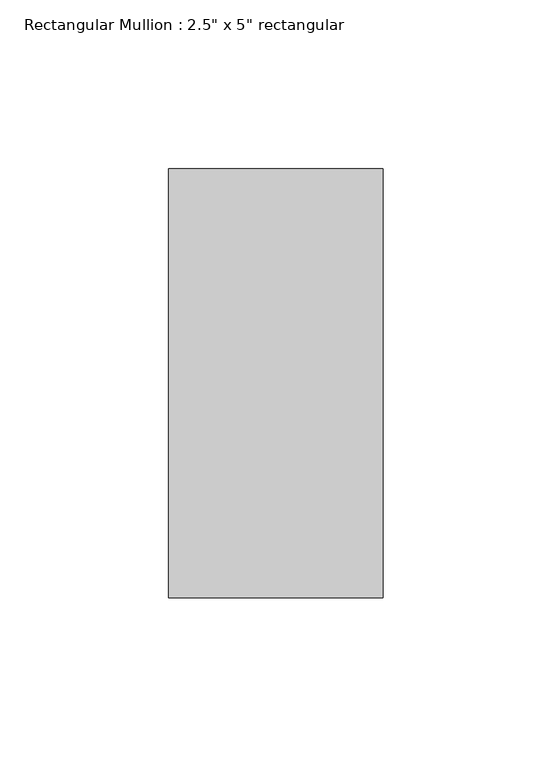
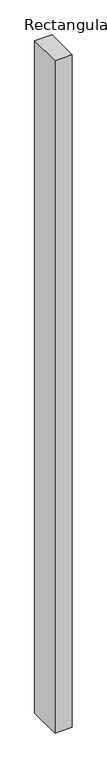
"""IFC4 building model written with IfcOpenShell, lengths in millimetres: member geometry."""

from ifc_helpers import new_model, si_unit, frame, origin, place, context, project, spatial, polyline, outline, extrude, source, transform, mapped, element, save


def member_3e16bac7(model_context):
    return source(origin(), model_context, "Body", "SweptSolid", [
        extrude(outline(polyline([(0.0, 63.5), (0.0, -63.5), (-63.5, -63.5), (-63.5, 63.5), (0.0, 63.5)])), frame((0.0, 0.0, -2587.728654), z_axis=(0.0, 0.0, 1.0), x_axis=(1.0, 0.0, 0.0)), (0.0, 0.0, 1.0), 2587.728654),
    ])


if __name__ == "__main__":
    model = new_model("IFC4")
    model_context = context("Model", 3, world=origin())
    ifc_project = project(units=[si_unit("LENGTHUNIT", "METRE", prefix="MILLI")], contexts=[model_context])
    site = spatial("IfcSite", under=ifc_project)
    building = spatial("IfcBuilding", under=site)
    placement = place(None, origin())
    member_shape = member_3e16bac7(model_context)
    element("IfcMember", 1, ObjectType="Rectangular Mullion : 2.5\" x 5\" rectangular", at=placement, inside=building, context=model_context, shape_type="MappedRepresentation", body=[
        mapped(member_shape, transform((0.0, 0.0, 0.0), x_axis=(1.0, 0.0, 0.0), y_axis=(0.0, 1.0, 0.0), z_axis=(0.0, 0.0, 1.0))),
    ])
    save(model, "model.ifc")

# Revit data of these elements
# Type "Rectangular Mullion : 2.5\" x 5\" rectangular"
#   built-in parameter 1007304 = 0.416667 (stored number, unit not read)
#   built-in parameter 1007301 = 0.104167 (stored number, unit not read)
#   built-in parameter 1007300 = 0.104167 (stored number, unit not read)
# Element 1 (IfcMember, "Rectangular Mullion : 2.5\" x 5\" rectangular")
#   Materials on its faces: "Aluminum"
# Materials
#   "Aluminum": class "Metal", colour RGB 247 247 247, transparency 0, Description = "Aluminum 6061", Cost = 0
